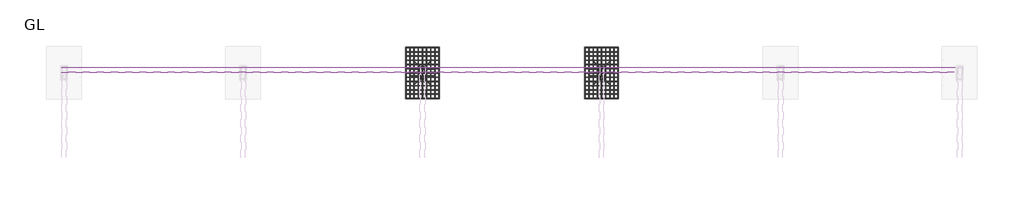
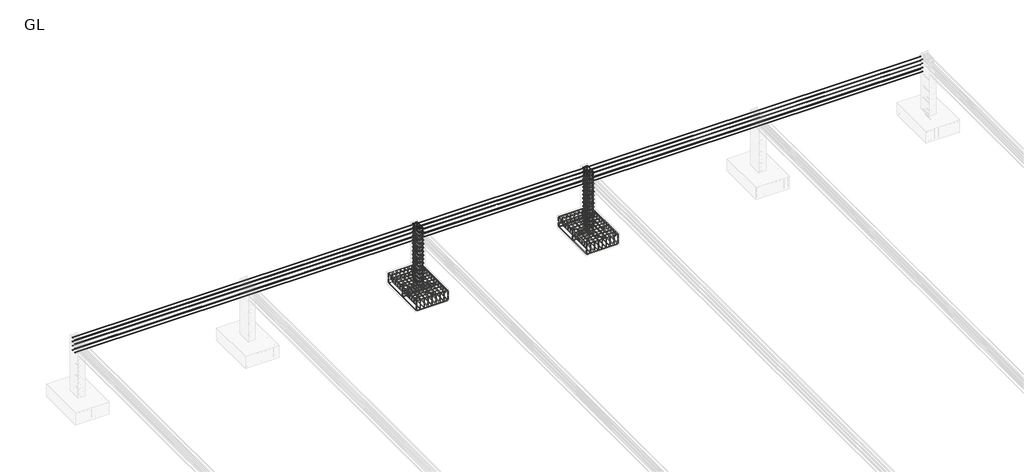
# One storey, part 15 of 16: 23 reinforcing bars.
"""IFC4 building model written with IfcOpenShell, lengths in millimetres."""

from ifc_helpers import new_model, si_unit, point, frame, origin, place, context, project, spatial, polyline, circle_curve, trimmed, segment, composite_curve, source, transform, mapped, element, save
from ifc_brep_helpers import swept_disk

model = new_model("IFC4")

# Units and contexts
model_context = context("Model", 3, world=origin())
ifc_project = project(units=[si_unit("LENGTHUNIT", "METRE", prefix="MILLI")], contexts=[model_context])

# Site, building, storey
site = spatial("IfcSite", under=ifc_project)
building = spatial("IfcBuilding", under=site)
storey = spatial("IfcBuildingStorey", under=building, Name="GL", Elevation=-1829.0)

# Reinforcing bars
placement = place(None, origin())
reinforcing_bar_shape = source(origin(), model_context, "Body", "SolidModel", [
    swept_disk(composite_curve([segment(polyline([(-10050.9544379, 4968.8832479, -2089.0), (-10050.9544379, 4968.8832479, -2213.0)]), True, "CONTINUOUS"), segment(trimmed(circle_curve(frame((-10080.9544379, 4968.8832479, -2213.0), z_axis=(0.0, 1.0, 0.0), x_axis=(30.0, 0.0, 0.0)), 30.0), [point((-10050.9544379, 4968.8832479, -2213.0))], [point((-10080.9544379, 4968.8832479, -2243.0))], True, "CARTESIAN"), True, "CONTINUOUS"), segment(polyline([(-10080.9544379, 4968.8832479, -2243.0), (-11148.9544379, 4968.8832479, -2243.0)]), True, "CONTINUOUS"), segment(trimmed(circle_curve(frame((-11148.9544379, 4968.8832479, -2213.0), z_axis=(0.0, 1.0, 0.0), x_axis=(0.0, 0.0, -30.0)), 30.0), [point((-11148.9544379, 4968.8832479, -2243.0))], [point((-11178.9544379, 4968.8832479, -2213.0))], True, "CARTESIAN"), True, "CONTINUOUS"), segment(polyline([(-11178.9544379, 4968.8832479, -2213.0), (-11178.9544379, 4968.8832479, -2089.0)]), True, "CONTINUOUS")], self_intersect=False), 6.0),
])
element("IfcReinforcingBar", 1, at=placement, inside=storey, context=model_context, shape_type="MappedRepresentation", body=[
    mapped(reinforcing_bar_shape, transform((0.0, 0.0, 0.0), x_axis=(1.0, 0.0, 0.0), y_axis=(0.0, 1.0, 0.0), z_axis=(0.0, 0.0, 1.0))),
    mapped(reinforcing_bar_shape, transform((0.0, -864.0, 0.0), x_axis=(1.0, 0.0, 0.0), y_axis=(0.0, 1.0, 0.0), z_axis=(0.0, 0.0, 1.0))),
    mapped(reinforcing_bar_shape, transform((0.0, -1728.0, 0.0), x_axis=(1.0, 0.0, 0.0), y_axis=(0.0, 1.0, 0.0), z_axis=(0.0, 0.0, 1.0))),
])
reinforcing_bar_2_shape = source(origin(), model_context, "Body", "SolidModel", [
    swept_disk(composite_curve([segment(polyline([(-11178.9544379, 4968.8832479, -2022.436678), (-11178.9544379, 4968.8832479, -1898.436678)]), True, "CONTINUOUS"), segment(trimmed(circle_curve(frame((-11148.9544379, 4968.8832479, -1898.436678), z_axis=(0.0, 1.0, 0.0), x_axis=(-30.0, 0.0, 0.0)), 30.0), [point((-11178.9544379, 4968.8832479, -1898.436678))], [point((-11148.9544379, 4968.8832479, -1868.436678))], True, "CARTESIAN"), True, "CONTINUOUS"), segment(polyline([(-11148.9544379, 4968.8832479, -1868.436678), (-10080.9544379, 4968.8832479, -1868.436678)]), True, "CONTINUOUS"), segment(trimmed(circle_curve(frame((-10080.9544379, 4968.8832479, -1898.436678), z_axis=(0.0, 1.0, 0.0), x_axis=(0.0, 0.0, 30.0)), 30.0), [point((-10080.9544379, 4968.8832479, -1868.436678))], [point((-10050.9544379, 4968.8832479, -1898.436678))], True, "CARTESIAN"), True, "CONTINUOUS"), segment(polyline([(-10050.9544379, 4968.8832479, -1898.436678), (-10050.9544379, 4968.8832479, -2022.436678)]), True, "CONTINUOUS")], self_intersect=False), 6.0),
])
element("IfcReinforcingBar", 2, at=placement, inside=storey, context=model_context, shape_type="MappedRepresentation", body=[
    mapped(reinforcing_bar_2_shape, transform((0.0, 0.0, 0.0), x_axis=(1.0, 0.0, 0.0), y_axis=(0.0, 1.0, 0.0), z_axis=(0.0, 0.0, 1.0))),
    mapped(reinforcing_bar_2_shape, transform((0.0, -144.0, 0.0), x_axis=(1.0, 0.0, 0.0), y_axis=(0.0, 1.0, 0.0), z_axis=(0.0, 0.0, 1.0))),
    mapped(reinforcing_bar_2_shape, transform((0.0, -288.0, 0.0), x_axis=(1.0, 0.0, 0.0), y_axis=(0.0, 1.0, 0.0), z_axis=(0.0, 0.0, 1.0))),
    mapped(reinforcing_bar_2_shape, transform((0.0, -432.0, 0.0), x_axis=(1.0, 0.0, 0.0), y_axis=(0.0, 1.0, 0.0), z_axis=(0.0, 0.0, 1.0))),
    mapped(reinforcing_bar_2_shape, transform((0.0, -576.0, 0.0), x_axis=(1.0, 0.0, 0.0), y_axis=(0.0, 1.0, 0.0), z_axis=(0.0, 0.0, 1.0))),
    mapped(reinforcing_bar_2_shape, transform((0.0, -720.0, 0.0), x_axis=(1.0, 0.0, 0.0), y_axis=(0.0, 1.0, 0.0), z_axis=(0.0, 0.0, 1.0))),
    mapped(reinforcing_bar_2_shape, transform((0.0, -864.0, 0.0), x_axis=(1.0, 0.0, 0.0), y_axis=(0.0, 1.0, 0.0), z_axis=(0.0, 0.0, 1.0))),
    mapped(reinforcing_bar_2_shape, transform((0.0, -1008.0, 0.0), x_axis=(1.0, 0.0, 0.0), y_axis=(0.0, 1.0, 0.0), z_axis=(0.0, 0.0, 1.0))),
    mapped(reinforcing_bar_2_shape, transform((0.0, -1152.0, 0.0), x_axis=(1.0, 0.0, 0.0), y_axis=(0.0, 1.0, 0.0), z_axis=(0.0, 0.0, 1.0))),
    mapped(reinforcing_bar_2_shape, transform((0.0, -1296.0, 0.0), x_axis=(1.0, 0.0, 0.0), y_axis=(0.0, 1.0, 0.0), z_axis=(0.0, 0.0, 1.0))),
    mapped(reinforcing_bar_2_shape, transform((0.0, -1440.0, 0.0), x_axis=(1.0, 0.0, 0.0), y_axis=(0.0, 1.0, 0.0), z_axis=(0.0, 0.0, 1.0))),
    mapped(reinforcing_bar_2_shape, transform((0.0, -1584.0, 0.0), x_axis=(1.0, 0.0, 0.0), y_axis=(0.0, 1.0, 0.0), z_axis=(0.0, 0.0, 1.0))),
    mapped(reinforcing_bar_2_shape, transform((0.0, -1728.0, 0.0), x_axis=(1.0, 0.0, 0.0), y_axis=(0.0, 1.0, 0.0), z_axis=(0.0, 0.0, 1.0))),
])
reinforcing_bar_3_shape = source(origin(), model_context, "Body", "SolidModel", [
    swept_disk(composite_curve([segment(polyline([(-11178.9544379, 3240.8832479, -2027.5081232), (-11178.9544379, 3240.8832479, -1903.5081232)]), True, "CONTINUOUS"), segment(trimmed(circle_curve(frame((-11178.9544379, 3270.8832479, -1903.5081232), z_axis=(-1.0, 0.0, 0.0), x_axis=(0.0, -30.0, 0.0)), 30.0), [point((-11178.9544379, 3240.8832479, -1903.5081232))], [point((-11178.9544379, 3270.8832479, -1873.5081232))], True, "CARTESIAN"), True, "CONTINUOUS"), segment(polyline([(-11178.9544379, 3270.8832479, -1873.5081232), (-11178.9544379, 4938.8832479, -1873.5081232)]), True, "CONTINUOUS"), segment(trimmed(circle_curve(frame((-11178.9544379, 4938.8832479, -1903.5081232), z_axis=(-1.0, 0.0, 0.0), x_axis=(0.0, 0.0, 30.0)), 30.0), [point((-11178.9544379, 4938.8832479, -1873.5081232))], [point((-11178.9544379, 4968.8832479, -1903.5081232))], True, "CARTESIAN"), True, "CONTINUOUS"), segment(polyline([(-11178.9544379, 4968.8832479, -1903.5081232), (-11178.9544379, 4968.8832479, -2027.5081232)]), True, "CONTINUOUS")], self_intersect=False), 6.0),
])
element("IfcReinforcingBar", 3, at=placement, inside=storey, context=model_context, shape_type="MappedRepresentation", body=[
    mapped(reinforcing_bar_3_shape, transform((0.0, 0.0, 0.0), x_axis=(1.0, 0.0, 0.0), y_axis=(0.0, 1.0, 0.0), z_axis=(0.0, 0.0, 1.0))),
    mapped(reinforcing_bar_3_shape, transform((141.0, 0.0, 0.0), x_axis=(1.0, 0.0, 0.0), y_axis=(0.0, 1.0, 0.0), z_axis=(0.0, 0.0, 1.0))),
    mapped(reinforcing_bar_3_shape, transform((282.0, 0.0, 0.0), x_axis=(1.0, 0.0, 0.0), y_axis=(0.0, 1.0, 0.0), z_axis=(0.0, 0.0, 1.0))),
    mapped(reinforcing_bar_3_shape, transform((423.0, 0.0, 0.0), x_axis=(1.0, 0.0, 0.0), y_axis=(0.0, 1.0, 0.0), z_axis=(0.0, 0.0, 1.0))),
    mapped(reinforcing_bar_3_shape, transform((564.0, 0.0, 0.0), x_axis=(1.0, 0.0, 0.0), y_axis=(0.0, 1.0, 0.0), z_axis=(0.0, 0.0, 1.0))),
    mapped(reinforcing_bar_3_shape, transform((705.0, 0.0, 0.0), x_axis=(1.0, 0.0, 0.0), y_axis=(0.0, 1.0, 0.0), z_axis=(0.0, 0.0, 1.0))),
    mapped(reinforcing_bar_3_shape, transform((846.0, 0.0, 0.0), x_axis=(1.0, 0.0, 0.0), y_axis=(0.0, 1.0, 0.0), z_axis=(0.0, 0.0, 1.0))),
    mapped(reinforcing_bar_3_shape, transform((987.0, 0.0, 0.0), x_axis=(1.0, 0.0, 0.0), y_axis=(0.0, 1.0, 0.0), z_axis=(0.0, 0.0, 1.0))),
    mapped(reinforcing_bar_3_shape, transform((1128.0, 0.0, 0.0), x_axis=(1.0, 0.0, 0.0), y_axis=(0.0, 1.0, 0.0), z_axis=(0.0, 0.0, 1.0))),
])
reinforcing_bar_4_shape = source(origin(), model_context, "Body", "SolidModel", [
    swept_disk(composite_curve([segment(polyline([(-10050.9544379, 3240.8832479, -2080.6239909), (-10050.9544379, 3240.8832479, -2204.6239909)]), True, "CONTINUOUS"), segment(trimmed(circle_curve(frame((-10050.9544379, 3270.8832479, -2204.6239909), z_axis=(1.0, 0.0, 0.0), x_axis=(0.0, -30.0, 0.0)), 30.0), [point((-10050.9544379, 3240.8832479, -2204.6239909))], [point((-10050.9544379, 3270.8832479, -2234.6239909))], True, "CARTESIAN"), True, "CONTINUOUS"), segment(polyline([(-10050.9544379, 3270.8832479, -2234.6239909), (-10050.9544379, 4925.8578108, -2234.6239909)]), True, "CONTINUOUS"), segment(trimmed(circle_curve(frame((-10050.9544379, 4925.8578108, -2204.6239909), z_axis=(1.0, 0.0, 0.0), x_axis=(0.0, 0.0, -30.0)), 30.0), [point((-10050.9544379, 4925.8578108, -2234.6239909))], [point((-10050.9544379, 4955.8578108, -2204.6239909))], True, "CARTESIAN"), True, "CONTINUOUS"), segment(polyline([(-10050.9544379, 4955.8578108, -2204.6239909), (-10050.9544379, 4955.8578108, -2080.6239909)]), True, "CONTINUOUS")], self_intersect=False), 6.0),
])
element("IfcReinforcingBar", 4, at=placement, inside=storey, context=model_context, shape_type="MappedRepresentation", body=[
    mapped(reinforcing_bar_4_shape, transform((0.0, 0.0, 0.0), x_axis=(1.0, 0.0, 0.0), y_axis=(0.0, 1.0, 0.0), z_axis=(0.0, 0.0, 1.0))),
    mapped(reinforcing_bar_4_shape, transform((-141.0, 0.0, 0.0), x_axis=(1.0, 0.0, 0.0), y_axis=(0.0, 1.0, 0.0), z_axis=(0.0, 0.0, 1.0))),
    mapped(reinforcing_bar_4_shape, transform((-282.0, 0.0, 0.0), x_axis=(1.0, 0.0, 0.0), y_axis=(0.0, 1.0, 0.0), z_axis=(0.0, 0.0, 1.0))),
    mapped(reinforcing_bar_4_shape, transform((-423.0, 0.0, 0.0), x_axis=(1.0, 0.0, 0.0), y_axis=(0.0, 1.0, 0.0), z_axis=(0.0, 0.0, 1.0))),
    mapped(reinforcing_bar_4_shape, transform((-564.0, 0.0, 0.0), x_axis=(1.0, 0.0, 0.0), y_axis=(0.0, 1.0, 0.0), z_axis=(0.0, 0.0, 1.0))),
    mapped(reinforcing_bar_4_shape, transform((-705.0, 0.0, 0.0), x_axis=(1.0, 0.0, 0.0), y_axis=(0.0, 1.0, 0.0), z_axis=(0.0, 0.0, 1.0))),
    mapped(reinforcing_bar_4_shape, transform((-846.0, 0.0, 0.0), x_axis=(1.0, 0.0, 0.0), y_axis=(0.0, 1.0, 0.0), z_axis=(0.0, 0.0, 1.0))),
    mapped(reinforcing_bar_4_shape, transform((-987.0, 0.0, 0.0), x_axis=(1.0, 0.0, 0.0), y_axis=(0.0, 1.0, 0.0), z_axis=(0.0, 0.0, 1.0))),
    mapped(reinforcing_bar_4_shape, transform((-1128.0, 0.0, 0.0), x_axis=(1.0, 0.0, 0.0), y_axis=(0.0, 1.0, 0.0), z_axis=(0.0, 0.0, 1.0))),
])
reinforcing_bar_5_shape = source(origin(), model_context, "Body", "SolidModel", [
    swept_disk(composite_curve([segment(polyline([(-3954.9544379, 4968.8832479, -2089.0), (-3954.9544379, 4968.8832479, -2213.0)]), True, "CONTINUOUS"), segment(trimmed(circle_curve(frame((-3984.9544379, 4968.8832479, -2213.0), z_axis=(0.0, 1.0, 0.0), x_axis=(30.0, 0.0, 0.0)), 30.0), [point((-3954.9544379, 4968.8832479, -2213.0))], [point((-3984.9544379, 4968.8832479, -2243.0))], True, "CARTESIAN"), True, "CONTINUOUS"), segment(polyline([(-3984.9544379, 4968.8832479, -2243.0), (-5052.9544379, 4968.8832479, -2243.0)]), True, "CONTINUOUS"), segment(trimmed(circle_curve(frame((-5052.9544379, 4968.8832479, -2213.0), z_axis=(0.0, 1.0, 0.0), x_axis=(0.0, 0.0, -30.0)), 30.0), [point((-5052.9544379, 4968.8832479, -2243.0))], [point((-5082.9544379, 4968.8832479, -2213.0))], True, "CARTESIAN"), True, "CONTINUOUS"), segment(polyline([(-5082.9544379, 4968.8832479, -2213.0), (-5082.9544379, 4968.8832479, -2089.0)]), True, "CONTINUOUS")], self_intersect=False), 6.0),
])
element("IfcReinforcingBar", 5, at=placement, inside=storey, context=model_context, shape_type="MappedRepresentation", body=[
    mapped(reinforcing_bar_5_shape, transform((0.0, 0.0, 0.0), x_axis=(1.0, 0.0, 0.0), y_axis=(0.0, 1.0, 0.0), z_axis=(0.0, 0.0, 1.0))),
    mapped(reinforcing_bar_5_shape, transform((0.0, -864.0, 0.0), x_axis=(1.0, 0.0, 0.0), y_axis=(0.0, 1.0, 0.0), z_axis=(0.0, 0.0, 1.0))),
    mapped(reinforcing_bar_5_shape, transform((0.0, -1728.0, 0.0), x_axis=(1.0, 0.0, 0.0), y_axis=(0.0, 1.0, 0.0), z_axis=(0.0, 0.0, 1.0))),
])
reinforcing_bar_6_shape = source(origin(), model_context, "Body", "SolidModel", [
    swept_disk(composite_curve([segment(polyline([(-5082.9544379, 4968.8832479, -2022.436678), (-5082.9544379, 4968.8832479, -1898.436678)]), True, "CONTINUOUS"), segment(trimmed(circle_curve(frame((-5052.9544379, 4968.8832479, -1898.436678), z_axis=(0.0, 1.0, 0.0), x_axis=(-30.0, 0.0, 0.0)), 30.0), [point((-5082.9544379, 4968.8832479, -1898.436678))], [point((-5052.9544379, 4968.8832479, -1868.436678))], True, "CARTESIAN"), True, "CONTINUOUS"), segment(polyline([(-5052.9544379, 4968.8832479, -1868.436678), (-3984.9544379, 4968.8832479, -1868.436678)]), True, "CONTINUOUS"), segment(trimmed(circle_curve(frame((-3984.9544379, 4968.8832479, -1898.436678), z_axis=(0.0, 1.0, 0.0), x_axis=(0.0, 0.0, 30.0)), 30.0), [point((-3984.9544379, 4968.8832479, -1868.436678))], [point((-3954.9544379, 4968.8832479, -1898.436678))], True, "CARTESIAN"), True, "CONTINUOUS"), segment(polyline([(-3954.9544379, 4968.8832479, -1898.436678), (-3954.9544379, 4968.8832479, -2022.436678)]), True, "CONTINUOUS")], self_intersect=False), 6.0),
])
element("IfcReinforcingBar", 6, at=placement, inside=storey, context=model_context, shape_type="MappedRepresentation", body=[
    mapped(reinforcing_bar_6_shape, transform((0.0, 0.0, 0.0), x_axis=(1.0, 0.0, 0.0), y_axis=(0.0, 1.0, 0.0), z_axis=(0.0, 0.0, 1.0))),
    mapped(reinforcing_bar_6_shape, transform((0.0, -144.0, 0.0), x_axis=(1.0, 0.0, 0.0), y_axis=(0.0, 1.0, 0.0), z_axis=(0.0, 0.0, 1.0))),
    mapped(reinforcing_bar_6_shape, transform((0.0, -288.0, 0.0), x_axis=(1.0, 0.0, 0.0), y_axis=(0.0, 1.0, 0.0), z_axis=(0.0, 0.0, 1.0))),
    mapped(reinforcing_bar_6_shape, transform((0.0, -432.0, 0.0), x_axis=(1.0, 0.0, 0.0), y_axis=(0.0, 1.0, 0.0), z_axis=(0.0, 0.0, 1.0))),
    mapped(reinforcing_bar_6_shape, transform((0.0, -576.0, 0.0), x_axis=(1.0, 0.0, 0.0), y_axis=(0.0, 1.0, 0.0), z_axis=(0.0, 0.0, 1.0))),
    mapped(reinforcing_bar_6_shape, transform((0.0, -720.0, 0.0), x_axis=(1.0, 0.0, 0.0), y_axis=(0.0, 1.0, 0.0), z_axis=(0.0, 0.0, 1.0))),
    mapped(reinforcing_bar_6_shape, transform((0.0, -864.0, 0.0), x_axis=(1.0, 0.0, 0.0), y_axis=(0.0, 1.0, 0.0), z_axis=(0.0, 0.0, 1.0))),
    mapped(reinforcing_bar_6_shape, transform((0.0, -1008.0, 0.0), x_axis=(1.0, 0.0, 0.0), y_axis=(0.0, 1.0, 0.0), z_axis=(0.0, 0.0, 1.0))),
    mapped(reinforcing_bar_6_shape, transform((0.0, -1152.0, 0.0), x_axis=(1.0, 0.0, 0.0), y_axis=(0.0, 1.0, 0.0), z_axis=(0.0, 0.0, 1.0))),
    mapped(reinforcing_bar_6_shape, transform((0.0, -1296.0, 0.0), x_axis=(1.0, 0.0, 0.0), y_axis=(0.0, 1.0, 0.0), z_axis=(0.0, 0.0, 1.0))),
    mapped(reinforcing_bar_6_shape, transform((0.0, -1440.0, 0.0), x_axis=(1.0, 0.0, 0.0), y_axis=(0.0, 1.0, 0.0), z_axis=(0.0, 0.0, 1.0))),
    mapped(reinforcing_bar_6_shape, transform((0.0, -1584.0, 0.0), x_axis=(1.0, 0.0, 0.0), y_axis=(0.0, 1.0, 0.0), z_axis=(0.0, 0.0, 1.0))),
    mapped(reinforcing_bar_6_shape, transform((0.0, -1728.0, 0.0), x_axis=(1.0, 0.0, 0.0), y_axis=(0.0, 1.0, 0.0), z_axis=(0.0, 0.0, 1.0))),
])
reinforcing_bar_7_shape = source(origin(), model_context, "Body", "SolidModel", [
    swept_disk(composite_curve([segment(polyline([(-5082.9544379, 3240.8832479, -2027.5081232), (-5082.9544379, 3240.8832479, -1903.5081232)]), True, "CONTINUOUS"), segment(trimmed(circle_curve(frame((-5082.9544379, 3270.8832479, -1903.5081232), z_axis=(-1.0, 0.0, 0.0), x_axis=(0.0, -30.0, 0.0)), 30.0), [point((-5082.9544379, 3240.8832479, -1903.5081232))], [point((-5082.9544379, 3270.8832479, -1873.5081232))], True, "CARTESIAN"), True, "CONTINUOUS"), segment(polyline([(-5082.9544379, 3270.8832479, -1873.5081232), (-5082.9544379, 4938.8832479, -1873.5081232)]), True, "CONTINUOUS"), segment(trimmed(circle_curve(frame((-5082.9544379, 4938.8832479, -1903.5081232), z_axis=(-1.0, 0.0, 0.0), x_axis=(0.0, 0.0, 30.0)), 30.0), [point((-5082.9544379, 4938.8832479, -1873.5081232))], [point((-5082.9544379, 4968.8832479, -1903.5081232))], True, "CARTESIAN"), True, "CONTINUOUS"), segment(polyline([(-5082.9544379, 4968.8832479, -1903.5081232), (-5082.9544379, 4968.8832479, -2027.5081232)]), True, "CONTINUOUS")], self_intersect=False), 6.0),
])
element("IfcReinforcingBar", 7, at=placement, inside=storey, context=model_context, shape_type="MappedRepresentation", body=[
    mapped(reinforcing_bar_7_shape, transform((0.0, 0.0, 0.0), x_axis=(1.0, 0.0, 0.0), y_axis=(0.0, 1.0, 0.0), z_axis=(0.0, 0.0, 1.0))),
    mapped(reinforcing_bar_7_shape, transform((141.0, 0.0, 0.0), x_axis=(1.0, 0.0, 0.0), y_axis=(0.0, 1.0, 0.0), z_axis=(0.0, 0.0, 1.0))),
    mapped(reinforcing_bar_7_shape, transform((282.0, 0.0, 0.0), x_axis=(1.0, 0.0, 0.0), y_axis=(0.0, 1.0, 0.0), z_axis=(0.0, 0.0, 1.0))),
    mapped(reinforcing_bar_7_shape, transform((423.0, 0.0, 0.0), x_axis=(1.0, 0.0, 0.0), y_axis=(0.0, 1.0, 0.0), z_axis=(0.0, 0.0, 1.0))),
    mapped(reinforcing_bar_7_shape, transform((564.0, 0.0, 0.0), x_axis=(1.0, 0.0, 0.0), y_axis=(0.0, 1.0, 0.0), z_axis=(0.0, 0.0, 1.0))),
    mapped(reinforcing_bar_7_shape, transform((705.0, 0.0, 0.0), x_axis=(1.0, 0.0, 0.0), y_axis=(0.0, 1.0, 0.0), z_axis=(0.0, 0.0, 1.0))),
    mapped(reinforcing_bar_7_shape, transform((846.0, 0.0, 0.0), x_axis=(1.0, 0.0, 0.0), y_axis=(0.0, 1.0, 0.0), z_axis=(0.0, 0.0, 1.0))),
    mapped(reinforcing_bar_7_shape, transform((987.0, 0.0, 0.0), x_axis=(1.0, 0.0, 0.0), y_axis=(0.0, 1.0, 0.0), z_axis=(0.0, 0.0, 1.0))),
    mapped(reinforcing_bar_7_shape, transform((1128.0, 0.0, 0.0), x_axis=(1.0, 0.0, 0.0), y_axis=(0.0, 1.0, 0.0), z_axis=(0.0, 0.0, 1.0))),
])
reinforcing_bar_8_shape = source(origin(), model_context, "Body", "SolidModel", [
    swept_disk(composite_curve([segment(polyline([(-3954.9544379, 3240.8832479, -2080.6239909), (-3954.9544379, 3240.8832479, -2204.6239909)]), True, "CONTINUOUS"), segment(trimmed(circle_curve(frame((-3954.9544379, 3270.8832479, -2204.6239909), z_axis=(1.0, 0.0, 0.0), x_axis=(0.0, -30.0, 0.0)), 30.0), [point((-3954.9544379, 3240.8832479, -2204.6239909))], [point((-3954.9544379, 3270.8832479, -2234.6239909))], True, "CARTESIAN"), True, "CONTINUOUS"), segment(polyline([(-3954.9544379, 3270.8832479, -2234.6239909), (-3954.9544379, 4925.8578108, -2234.6239909)]), True, "CONTINUOUS"), segment(trimmed(circle_curve(frame((-3954.9544379, 4925.8578108, -2204.6239909), z_axis=(1.0, 0.0, 0.0), x_axis=(0.0, 0.0, -30.0)), 30.0), [point((-3954.9544379, 4925.8578108, -2234.6239909))], [point((-3954.9544379, 4955.8578108, -2204.6239909))], True, "CARTESIAN"), True, "CONTINUOUS"), segment(polyline([(-3954.9544379, 4955.8578108, -2204.6239909), (-3954.9544379, 4955.8578108, -2080.6239909)]), True, "CONTINUOUS")], self_intersect=False), 6.0),
])
element("IfcReinforcingBar", 8, at=placement, inside=storey, context=model_context, shape_type="MappedRepresentation", body=[
    mapped(reinforcing_bar_8_shape, transform((0.0, 0.0, 0.0), x_axis=(1.0, 0.0, 0.0), y_axis=(0.0, 1.0, 0.0), z_axis=(0.0, 0.0, 1.0))),
    mapped(reinforcing_bar_8_shape, transform((-141.0, 0.0, 0.0), x_axis=(1.0, 0.0, 0.0), y_axis=(0.0, 1.0, 0.0), z_axis=(0.0, 0.0, 1.0))),
    mapped(reinforcing_bar_8_shape, transform((-282.0, 0.0, 0.0), x_axis=(1.0, 0.0, 0.0), y_axis=(0.0, 1.0, 0.0), z_axis=(0.0, 0.0, 1.0))),
    mapped(reinforcing_bar_8_shape, transform((-423.0, 0.0, 0.0), x_axis=(1.0, 0.0, 0.0), y_axis=(0.0, 1.0, 0.0), z_axis=(0.0, 0.0, 1.0))),
    mapped(reinforcing_bar_8_shape, transform((-564.0, 0.0, 0.0), x_axis=(1.0, 0.0, 0.0), y_axis=(0.0, 1.0, 0.0), z_axis=(0.0, 0.0, 1.0))),
    mapped(reinforcing_bar_8_shape, transform((-705.0, 0.0, 0.0), x_axis=(1.0, 0.0, 0.0), y_axis=(0.0, 1.0, 0.0), z_axis=(0.0, 0.0, 1.0))),
    mapped(reinforcing_bar_8_shape, transform((-846.0, 0.0, 0.0), x_axis=(1.0, 0.0, 0.0), y_axis=(0.0, 1.0, 0.0), z_axis=(0.0, 0.0, 1.0))),
    mapped(reinforcing_bar_8_shape, transform((-987.0, 0.0, 0.0), x_axis=(1.0, 0.0, 0.0), y_axis=(0.0, 1.0, 0.0), z_axis=(0.0, 0.0, 1.0))),
    mapped(reinforcing_bar_8_shape, transform((-1128.0, 0.0, 0.0), x_axis=(1.0, 0.0, 0.0), y_axis=(0.0, 1.0, 0.0), z_axis=(0.0, 0.0, 1.0))),
])
reinforcing_bar_9_shape = source(origin(), model_context, "Body", "SolidModel", [
    swept_disk(composite_curve([segment(polyline([(-10607.4864005, 4029.7776922, -1793.0), (-10695.1676414, 3942.0964514, -1793.0)]), True, "CONTINUOUS"), segment(trimmed(circle_curve(frame((-10673.9544379, 3920.8832479, -1793.0), z_axis=(0.0, 0.0, 1.0), x_axis=(-21.21320349999951, 21.213203500000418, 0.0)), 30.0), [point((-10695.1676414, 3942.0964514, -1793.0))], [point((-10673.9544379, 3890.8832479, -1793.0))], True, "CARTESIAN"), True, "CONTINUOUS"), segment(polyline([(-10673.9544379, 3890.8832479, -1793.0), (-10555.9544379, 3890.8832479, -1793.0)]), True, "CONTINUOUS"), segment(trimmed(circle_curve(frame((-10555.9544379, 3920.8832479, -1793.0), z_axis=(0.0, 0.0, 1.0), x_axis=(0.0, -30.0, 0.0)), 30.0), [point((-10555.9544379, 3890.8832479, -1793.0))], [point((-10525.9544379, 3920.8832479, -1793.0))], True, "CARTESIAN"), True, "CONTINUOUS"), segment(polyline([(-10525.9544379, 3920.8832479, -1793.0), (-10525.9544379, 4288.8832479, -1793.0)]), True, "CONTINUOUS"), segment(trimmed(circle_curve(frame((-10555.8864962, 4288.8832479, -1795.0178916), z_axis=(-0.06726305234213417, 0.0, 0.9977352764083365), x_axis=(29.93205830000079, 0.0, 2.0178915999999845)), 30.0), [point((-10525.9544379, 4288.8832479, -1793.0))], [point((-10555.8864962, 4318.8832479, -1795.0178916))], True, "CARTESIAN"), True, "CONTINUOUS"), segment(polyline([(-10555.8864962, 4318.8832479, -1795.0178916), (-10674.0223796, 4318.8832479, -1802.9821084)]), True, "CONTINUOUS"), segment(trimmed(circle_curve(frame((-10674.0223796, 4288.8832479, -1802.9821084), z_axis=(-0.06726305234213417, 0.0, 0.9977352764083365), x_axis=(0.0, 30.0, 0.0)), 30.0), [point((-10674.0223796, 4318.8832479, -1802.9821084))], [point((-10703.9544379, 4288.8832479, -1805.0))], True, "CARTESIAN"), True, "CONTINUOUS"), segment(polyline([(-10703.9544379, 4288.8832479, -1805.0), (-10703.9544379, 3920.8832479, -1805.0)]), True, "CONTINUOUS"), segment(trimmed(circle_curve(frame((-10673.9544379, 3920.8832479, -1805.0), z_axis=(0.0, 0.0, 1.0), x_axis=(-30.0, 0.0, 0.0)), 30.0), [point((-10703.9544379, 3920.8832479, -1805.0))], [point((-10652.7412345, 3899.6700445, -1805.0))], True, "CARTESIAN"), True, "CONTINUOUS"), segment(polyline([(-10652.7412345, 3899.6700445, -1805.0), (-10565.0599936, 3987.3512854, -1805.0)]), True, "CONTINUOUS")], self_intersect=False), 6.0),
])
element("IfcReinforcingBar", 9, at=placement, inside=storey, context=model_context, shape_type="MappedRepresentation", body=[
    mapped(reinforcing_bar_9_shape, transform((0.0, 0.0, 0.0), x_axis=(1.0, 0.0, 0.0), y_axis=(0.0, 1.0, 0.0), z_axis=(0.0, 0.0, 1.0))),
    mapped(reinforcing_bar_9_shape, transform((0.0, 0.0, 144.8571429), x_axis=(1.0, 0.0, 0.0), y_axis=(0.0, 1.0, 0.0), z_axis=(0.0, 0.0, 1.0))),
    mapped(reinforcing_bar_9_shape, transform((0.0, 0.0, 289.7142857), x_axis=(1.0, 0.0, 0.0), y_axis=(0.0, 1.0, 0.0), z_axis=(0.0, 0.0, 1.0))),
    mapped(reinforcing_bar_9_shape, transform((0.0, 0.0, 434.5714286), x_axis=(1.0, 0.0, 0.0), y_axis=(0.0, 1.0, 0.0), z_axis=(0.0, 0.0, 1.0))),
    mapped(reinforcing_bar_9_shape, transform((0.0, 0.0, 579.4285714), x_axis=(1.0, 0.0, 0.0), y_axis=(0.0, 1.0, 0.0), z_axis=(0.0, 0.0, 1.0))),
    mapped(reinforcing_bar_9_shape, transform((0.0, 0.0, 724.2857143), x_axis=(1.0, 0.0, 0.0), y_axis=(0.0, 1.0, 0.0), z_axis=(0.0, 0.0, 1.0))),
    mapped(reinforcing_bar_9_shape, transform((0.0, 0.0, 869.1428571), x_axis=(1.0, 0.0, 0.0), y_axis=(0.0, 1.0, 0.0), z_axis=(0.0, 0.0, 1.0))),
    mapped(reinforcing_bar_9_shape, transform((0.0, 0.0, 1014.0), x_axis=(1.0, 0.0, 0.0), y_axis=(0.0, 1.0, 0.0), z_axis=(0.0, 0.0, 1.0))),
    mapped(reinforcing_bar_9_shape, transform((0.0, 0.0, 1158.8571429), x_axis=(1.0, 0.0, 0.0), y_axis=(0.0, 1.0, 0.0), z_axis=(0.0, 0.0, 1.0))),
    mapped(reinforcing_bar_9_shape, transform((0.0, 0.0, 1303.7142857), x_axis=(1.0, 0.0, 0.0), y_axis=(0.0, 1.0, 0.0), z_axis=(0.0, 0.0, 1.0))),
    mapped(reinforcing_bar_9_shape, transform((0.0, 0.0, 1448.5714286), x_axis=(1.0, 0.0, 0.0), y_axis=(0.0, 1.0, 0.0), z_axis=(0.0, 0.0, 1.0))),
    mapped(reinforcing_bar_9_shape, transform((0.0, 0.0, 1593.4285714), x_axis=(1.0, 0.0, 0.0), y_axis=(0.0, 1.0, 0.0), z_axis=(0.0, 0.0, 1.0))),
    mapped(reinforcing_bar_9_shape, transform((0.0, 0.0, 1738.2857143), x_axis=(1.0, 0.0, 0.0), y_axis=(0.0, 1.0, 0.0), z_axis=(0.0, 0.0, 1.0))),
    mapped(reinforcing_bar_9_shape, transform((0.0, 0.0, 1883.1428571), x_axis=(1.0, 0.0, 0.0), y_axis=(0.0, 1.0, 0.0), z_axis=(0.0, 0.0, 1.0))),
    mapped(reinforcing_bar_9_shape, transform((0.0, 0.0, 2028.0), x_axis=(1.0, 0.0, 0.0), y_axis=(0.0, 1.0, 0.0), z_axis=(0.0, 0.0, 1.0))),
])
element("IfcReinforcingBar", 10, at=placement, inside=storey, context=model_context, shape_type="SolidModel", body=[
    swept_disk(composite_curve([segment(polyline([(-10672.0642232, 3919.9357561, 241.0), (-10672.0642232, 3919.9357561, -2129.0)]), True, "CONTINUOUS"), segment(trimmed(circle_curve(frame((-10693.2774266, 3898.7225527, -2129.0), z_axis=(-0.7071067811865187, 0.7071067811865764, 0.0), x_axis=(21.213203400000566, 21.21320340000011, 0.0)), 30.0), [point((-10672.0642232, 3919.9357561, -2129.0))], [point((-10693.2774266, 3898.7225527, -2159.0))], True, "CARTESIAN"), True, "CONTINUOUS"), segment(polyline([(-10693.2774266, 3898.7225527, -2159.0), (-10940.7648, 3651.2351793, -2159.0)]), True, "CONTINUOUS")], self_intersect=False), 6.0),
])
element("IfcReinforcingBar", 11, at=placement, inside=storey, context=model_context, shape_type="SolidModel", body=[
    swept_disk(composite_curve([segment(polyline([(-10672.0642232, 4289.8307397, 241.0), (-10672.0642232, 4289.8307397, -2129.0)]), True, "CONTINUOUS"), segment(trimmed(circle_curve(frame((-10693.2774266, 4311.0439432, -2129.0), z_axis=(0.7071067811865218, 0.7071067811865733, 0.0), x_axis=(21.213203400000566, -21.213203500000418, 0.0)), 30.0), [point((-10672.0642232, 4289.8307397, -2129.0))], [point((-10693.2774266, 4311.0439432, -2159.0))], True, "CARTESIAN"), True, "CONTINUOUS"), segment(polyline([(-10693.2774266, 4311.0439432, -2159.0), (-10940.7648, 4558.5313166, -2159.0)]), True, "CONTINUOUS")], self_intersect=False), 6.0),
])
element("IfcReinforcingBar", 12, at=placement, inside=storey, context=model_context, shape_type="SolidModel", body=[
    swept_disk(composite_curve([segment(polyline([(-10557.8446527, 3919.9357561, 241.0), (-10557.8446527, 3919.9357561, -2129.0)]), True, "CONTINUOUS"), segment(trimmed(circle_curve(frame((-10536.6314492, 3898.7225527, -2129.0), z_axis=(-0.7071067811865248, -0.7071067811865703, 0.0), x_axis=(-21.21320349999951, 21.21320340000011, 0.0)), 30.0), [point((-10557.8446527, 3919.9357561, -2129.0))], [point((-10536.6314492, 3898.7225527, -2159.0))], True, "CARTESIAN"), True, "CONTINUOUS"), segment(polyline([(-10536.6314492, 3898.7225527, -2159.0), (-10289.1440758, 3651.2351793, -2159.0)]), True, "CONTINUOUS")], self_intersect=False), 6.0),
])
element("IfcReinforcingBar", 13, at=placement, inside=storey, context=model_context, shape_type="SolidModel", body=[
    swept_disk(composite_curve([segment(polyline([(-10557.8446527, 4289.8307397, 241.0), (-10557.8446527, 4289.8307397, -2129.0)]), True, "CONTINUOUS"), segment(trimmed(circle_curve(frame((-10536.6314492, 4311.0439432, -2129.0), z_axis=(0.7071067811865157, -0.7071067811865794, 0.0), x_axis=(-21.21320349999951, -21.213203500000418, 0.0)), 30.0), [point((-10557.8446527, 4289.8307397, -2129.0))], [point((-10536.6314492, 4311.0439432, -2159.0))], True, "CARTESIAN"), True, "CONTINUOUS"), segment(polyline([(-10536.6314492, 4311.0439432, -2159.0), (-10289.1440758, 4558.5313166, -2159.0)]), True, "CONTINUOUS")], self_intersect=False), 6.0),
])
reinforcing_bar_10_shape = source(origin(), model_context, "Body", "SolidModel", [
    swept_disk(composite_curve([segment(polyline([(-10672.0642232, 3997.0882595, 241.0), (-10672.0642232, 3997.0882595, -2129.0)]), True, "CONTINUOUS"), segment(trimmed(circle_curve(frame((-10702.0642232, 3997.0882595, -2129.0), z_axis=(0.0, 1.0, 0.0), x_axis=(30.0, 0.0, 0.0)), 30.0), [point((-10672.0642232, 3997.0882595, -2129.0))], [point((-10702.0642232, 3997.0882595, -2159.0))], True, "CARTESIAN"), True, "CONTINUOUS"), segment(polyline([(-10702.0642232, 3997.0882595, -2159.0), (-11052.0642232, 3997.0882595, -2159.0)]), True, "CONTINUOUS")], self_intersect=False), 6.0),
])
element("IfcReinforcingBar", 14, at=placement, inside=storey, context=model_context, shape_type="MappedRepresentation", body=[
    mapped(reinforcing_bar_10_shape, transform((0.0, 0.0, 0.0), x_axis=(1.0, 0.0, 0.0), y_axis=(0.0, 1.0, 0.0), z_axis=(0.0, 0.0, 1.0))),
    mapped(reinforcing_bar_10_shape, transform((0.0, 123.5823926, 0.0), x_axis=(1.0, 0.0, 0.0), y_axis=(0.0, 1.0, 0.0), z_axis=(0.0, 0.0, 1.0))),
    mapped(reinforcing_bar_10_shape, transform((0.0, 247.1647853, 0.0), x_axis=(1.0, 0.0, 0.0), y_axis=(0.0, 1.0, 0.0), z_axis=(0.0, 0.0, 1.0))),
])
reinforcing_bar_11_shape = source(origin(), model_context, "Body", "SolidModel", [
    swept_disk(composite_curve([segment(polyline([(-10557.8446527, 3997.0882595, 241.0), (-10557.8446527, 3997.0882595, -2129.0)]), True, "CONTINUOUS"), segment(trimmed(circle_curve(frame((-10527.8446527, 3997.0882595, -2129.0), z_axis=(0.0, -1.0, 0.0), x_axis=(-30.0, 0.0, 0.0)), 30.0), [point((-10557.8446527, 3997.0882595, -2129.0))], [point((-10527.8446527, 3997.0882595, -2159.0))], True, "CARTESIAN"), True, "CONTINUOUS"), segment(polyline([(-10527.8446527, 3997.0882595, -2159.0), (-10177.8446527, 3997.0882595, -2159.0)]), True, "CONTINUOUS")], self_intersect=False), 6.0),
])
element("IfcReinforcingBar", 15, at=placement, inside=storey, context=model_context, shape_type="MappedRepresentation", body=[
    mapped(reinforcing_bar_11_shape, transform((0.0, 0.0, 0.0), x_axis=(1.0, 0.0, 0.0), y_axis=(0.0, 1.0, 0.0), z_axis=(0.0, 0.0, 1.0))),
    mapped(reinforcing_bar_11_shape, transform((0.0, 123.5823926, 0.0), x_axis=(1.0, 0.0, 0.0), y_axis=(0.0, 1.0, 0.0), z_axis=(0.0, 0.0, 1.0))),
    mapped(reinforcing_bar_11_shape, transform((0.0, 247.1647853, 0.0), x_axis=(1.0, 0.0, 0.0), y_axis=(0.0, 1.0, 0.0), z_axis=(0.0, 0.0, 1.0))),
])
reinforcing_bar_12_shape = source(origin(), model_context, "Body", "SolidModel", [
    swept_disk(composite_curve([segment(polyline([(-4511.4864005, 4029.7776922, -1793.0), (-4599.1676414, 3942.0964514, -1793.0)]), True, "CONTINUOUS"), segment(trimmed(circle_curve(frame((-4577.9544379, 3920.8832479, -1793.0), z_axis=(0.0, 0.0, 1.0), x_axis=(-21.213203500000418, 21.213203500000418, 0.0)), 30.0), [point((-4599.1676414, 3942.0964514, -1793.0))], [point((-4577.9544379, 3890.8832479, -1793.0))], True, "CARTESIAN"), True, "CONTINUOUS"), segment(polyline([(-4577.9544379, 3890.8832479, -1793.0), (-4459.9544379, 3890.8832479, -1793.0)]), True, "CONTINUOUS"), segment(trimmed(circle_curve(frame((-4459.9544379, 3920.8832479, -1793.0), z_axis=(0.0, 0.0, 1.0), x_axis=(0.0, -30.0, 0.0)), 30.0), [point((-4459.9544379, 3890.8832479, -1793.0))], [point((-4429.9544379, 3920.8832479, -1793.0))], True, "CARTESIAN"), True, "CONTINUOUS"), segment(polyline([(-4429.9544379, 3920.8832479, -1793.0), (-4429.9544379, 4288.8832479, -1793.0)]), True, "CONTINUOUS"), segment(trimmed(circle_curve(frame((-4459.8864962, 4288.8832479, -1795.0178916), z_axis=(-0.06726305234213417, 0.0, 0.9977352764083365), x_axis=(29.93205829999988, 0.0, 2.0178915999999845)), 30.0), [point((-4429.9544379, 4288.8832479, -1793.0))], [point((-4459.8864962, 4318.8832479, -1795.0178916))], True, "CARTESIAN"), True, "CONTINUOUS"), segment(polyline([(-4459.8864962, 4318.8832479, -1795.0178916), (-4578.0223796, 4318.8832479, -1802.9821084)]), True, "CONTINUOUS"), segment(trimmed(circle_curve(frame((-4578.0223796, 4288.8832479, -1802.9821084), z_axis=(-0.06726305234213417, 0.0, 0.9977352764083365), x_axis=(0.0, 30.0, 0.0)), 30.0), [point((-4578.0223796, 4318.8832479, -1802.9821084))], [point((-4607.9544379, 4288.8832479, -1805.0))], True, "CARTESIAN"), True, "CONTINUOUS"), segment(polyline([(-4607.9544379, 4288.8832479, -1805.0), (-4607.9544379, 3920.8832479, -1805.0)]), True, "CONTINUOUS"), segment(trimmed(circle_curve(frame((-4577.9544379, 3920.8832479, -1805.0), z_axis=(0.0, 0.0, 1.0), x_axis=(-30.0, 0.0, 0.0)), 30.0), [point((-4607.9544379, 3920.8832479, -1805.0))], [point((-4556.7412345, 3899.6700445, -1805.0))], True, "CARTESIAN"), True, "CONTINUOUS"), segment(polyline([(-4556.7412345, 3899.6700445, -1805.0), (-4469.0599936, 3987.3512854, -1805.0)]), True, "CONTINUOUS")], self_intersect=False), 6.0),
])
element("IfcReinforcingBar", 16, at=placement, inside=storey, context=model_context, shape_type="MappedRepresentation", body=[
    mapped(reinforcing_bar_12_shape, transform((0.0, 0.0, 0.0), x_axis=(1.0, 0.0, 0.0), y_axis=(0.0, 1.0, 0.0), z_axis=(0.0, 0.0, 1.0))),
    mapped(reinforcing_bar_12_shape, transform((0.0, 0.0, 144.8571429), x_axis=(1.0, 0.0, 0.0), y_axis=(0.0, 1.0, 0.0), z_axis=(0.0, 0.0, 1.0))),
    mapped(reinforcing_bar_12_shape, transform((0.0, 0.0, 289.7142857), x_axis=(1.0, 0.0, 0.0), y_axis=(0.0, 1.0, 0.0), z_axis=(0.0, 0.0, 1.0))),
    mapped(reinforcing_bar_12_shape, transform((0.0, 0.0, 434.5714286), x_axis=(1.0, 0.0, 0.0), y_axis=(0.0, 1.0, 0.0), z_axis=(0.0, 0.0, 1.0))),
    mapped(reinforcing_bar_12_shape, transform((0.0, 0.0, 579.4285714), x_axis=(1.0, 0.0, 0.0), y_axis=(0.0, 1.0, 0.0), z_axis=(0.0, 0.0, 1.0))),
    mapped(reinforcing_bar_12_shape, transform((0.0, 0.0, 724.2857143), x_axis=(1.0, 0.0, 0.0), y_axis=(0.0, 1.0, 0.0), z_axis=(0.0, 0.0, 1.0))),
    mapped(reinforcing_bar_12_shape, transform((0.0, 0.0, 869.1428571), x_axis=(1.0, 0.0, 0.0), y_axis=(0.0, 1.0, 0.0), z_axis=(0.0, 0.0, 1.0))),
    mapped(reinforcing_bar_12_shape, transform((0.0, 0.0, 1014.0), x_axis=(1.0, 0.0, 0.0), y_axis=(0.0, 1.0, 0.0), z_axis=(0.0, 0.0, 1.0))),
    mapped(reinforcing_bar_12_shape, transform((0.0, 0.0, 1158.8571429), x_axis=(1.0, 0.0, 0.0), y_axis=(0.0, 1.0, 0.0), z_axis=(0.0, 0.0, 1.0))),
    mapped(reinforcing_bar_12_shape, transform((0.0, 0.0, 1303.7142857), x_axis=(1.0, 0.0, 0.0), y_axis=(0.0, 1.0, 0.0), z_axis=(0.0, 0.0, 1.0))),
    mapped(reinforcing_bar_12_shape, transform((0.0, 0.0, 1448.5714286), x_axis=(1.0, 0.0, 0.0), y_axis=(0.0, 1.0, 0.0), z_axis=(0.0, 0.0, 1.0))),
    mapped(reinforcing_bar_12_shape, transform((0.0, 0.0, 1593.4285714), x_axis=(1.0, 0.0, 0.0), y_axis=(0.0, 1.0, 0.0), z_axis=(0.0, 0.0, 1.0))),
    mapped(reinforcing_bar_12_shape, transform((0.0, 0.0, 1738.2857143), x_axis=(1.0, 0.0, 0.0), y_axis=(0.0, 1.0, 0.0), z_axis=(0.0, 0.0, 1.0))),
    mapped(reinforcing_bar_12_shape, transform((0.0, 0.0, 1883.1428571), x_axis=(1.0, 0.0, 0.0), y_axis=(0.0, 1.0, 0.0), z_axis=(0.0, 0.0, 1.0))),
    mapped(reinforcing_bar_12_shape, transform((0.0, 0.0, 2028.0), x_axis=(1.0, 0.0, 0.0), y_axis=(0.0, 1.0, 0.0), z_axis=(0.0, 0.0, 1.0))),
])
element("IfcReinforcingBar", 17, at=placement, inside=storey, context=model_context, shape_type="SolidModel", body=[
    swept_disk(composite_curve([segment(polyline([(-4576.0642232, 3919.9357561, 241.0), (-4576.0642232, 3919.9357561, -2129.0)]), True, "CONTINUOUS"), segment(trimmed(circle_curve(frame((-4597.2774266, 3898.7225527, -2129.0), z_axis=(-0.7071067811865187, 0.7071067811865764, 0.0), x_axis=(21.213203399999657, 21.21320340000011, 0.0)), 30.0), [point((-4576.0642232, 3919.9357561, -2129.0))], [point((-4597.2774266, 3898.7225527, -2159.0))], True, "CARTESIAN"), True, "CONTINUOUS"), segment(polyline([(-4597.2774266, 3898.7225527, -2159.0), (-4844.7648, 3651.2351793, -2159.0)]), True, "CONTINUOUS")], self_intersect=False), 6.0),
])
element("IfcReinforcingBar", 18, at=placement, inside=storey, context=model_context, shape_type="SolidModel", body=[
    swept_disk(composite_curve([segment(polyline([(-4576.0642232, 4289.8307397, 241.0), (-4576.0642232, 4289.8307397, -2129.0)]), True, "CONTINUOUS"), segment(trimmed(circle_curve(frame((-4597.2774266, 4311.0439432, -2129.0), z_axis=(0.7071067811865218, 0.7071067811865733, 0.0), x_axis=(21.213203399999657, -21.213203500000418, 0.0)), 30.0), [point((-4576.0642232, 4289.8307397, -2129.0))], [point((-4597.2774266, 4311.0439432, -2159.0))], True, "CARTESIAN"), True, "CONTINUOUS"), segment(polyline([(-4597.2774266, 4311.0439432, -2159.0), (-4844.7648, 4558.5313166, -2159.0)]), True, "CONTINUOUS")], self_intersect=False), 6.0),
])
element("IfcReinforcingBar", 19, at=placement, inside=storey, context=model_context, shape_type="SolidModel", body=[
    swept_disk(composite_curve([segment(polyline([(-4461.8446527, 3919.9357561, 241.0), (-4461.8446527, 3919.9357561, -2129.0)]), True, "CONTINUOUS"), segment(trimmed(circle_curve(frame((-4440.6314492, 3898.7225527, -2129.0), z_axis=(-0.7071067811865248, -0.7071067811865703, 0.0), x_axis=(-21.21320349999951, 21.21320340000011, 0.0)), 30.0), [point((-4461.8446527, 3919.9357561, -2129.0))], [point((-4440.6314492, 3898.7225527, -2159.0))], True, "CARTESIAN"), True, "CONTINUOUS"), segment(polyline([(-4440.6314492, 3898.7225527, -2159.0), (-4193.1440758, 3651.2351793, -2159.0)]), True, "CONTINUOUS")], self_intersect=False), 6.0),
])
element("IfcReinforcingBar", 20, at=placement, inside=storey, context=model_context, shape_type="SolidModel", body=[
    swept_disk(composite_curve([segment(polyline([(-4461.8446527, 4289.8307397, 241.0), (-4461.8446527, 4289.8307397, -2129.0)]), True, "CONTINUOUS"), segment(trimmed(circle_curve(frame((-4440.6314492, 4311.0439432, -2129.0), z_axis=(0.7071067811865157, -0.7071067811865794, 0.0), x_axis=(-21.21320349999951, -21.213203500000418, 0.0)), 30.0), [point((-4461.8446527, 4289.8307397, -2129.0))], [point((-4440.6314492, 4311.0439432, -2159.0))], True, "CARTESIAN"), True, "CONTINUOUS"), segment(polyline([(-4440.6314492, 4311.0439432, -2159.0), (-4193.1440758, 4558.5313166, -2159.0)]), True, "CONTINUOUS")], self_intersect=False), 6.0),
])
reinforcing_bar_13_shape = source(origin(), model_context, "Body", "SolidModel", [
    swept_disk(composite_curve([segment(polyline([(-4576.0642232, 3997.0882595, 241.0), (-4576.0642232, 3997.0882595, -2129.0)]), True, "CONTINUOUS"), segment(trimmed(circle_curve(frame((-4606.0642232, 3997.0882595, -2129.0), z_axis=(0.0, 1.0, 0.0), x_axis=(30.0, 0.0, 0.0)), 30.0), [point((-4576.0642232, 3997.0882595, -2129.0))], [point((-4606.0642232, 3997.0882595, -2159.0))], True, "CARTESIAN"), True, "CONTINUOUS"), segment(polyline([(-4606.0642232, 3997.0882595, -2159.0), (-4956.0642232, 3997.0882595, -2159.0)]), True, "CONTINUOUS")], self_intersect=False), 6.0),
])
element("IfcReinforcingBar", 21, at=placement, inside=storey, context=model_context, shape_type="MappedRepresentation", body=[
    mapped(reinforcing_bar_13_shape, transform((0.0, 0.0, 0.0), x_axis=(1.0, 0.0, 0.0), y_axis=(0.0, 1.0, 0.0), z_axis=(0.0, 0.0, 1.0))),
    mapped(reinforcing_bar_13_shape, transform((0.0, 123.5823926, 0.0), x_axis=(1.0, 0.0, 0.0), y_axis=(0.0, 1.0, 0.0), z_axis=(0.0, 0.0, 1.0))),
    mapped(reinforcing_bar_13_shape, transform((0.0, 247.1647853, 0.0), x_axis=(1.0, 0.0, 0.0), y_axis=(0.0, 1.0, 0.0), z_axis=(0.0, 0.0, 1.0))),
])
reinforcing_bar_14_shape = source(origin(), model_context, "Body", "SolidModel", [
    swept_disk(composite_curve([segment(polyline([(7496.2065564, 4288.0653602, 208.2829644), (-22901.9544379, 4288.0653602, 208.2829644)]), True, "CONTINUOUS")], self_intersect=False), 6.0),
])
element("IfcReinforcingBar", 22, at=placement, inside=storey, context=model_context, shape_type="MappedRepresentation", body=[
    mapped(reinforcing_bar_14_shape, transform((0.0, 0.0, 0.0), x_axis=(1.0, 0.0, 0.0), y_axis=(0.0, 1.0, 0.0), z_axis=(0.0, 0.0, 1.0))),
    mapped(reinforcing_bar_14_shape, transform((0.0, 0.0, -155.5868389), x_axis=(1.0, 0.0, 0.0), y_axis=(0.0, 1.0, 0.0), z_axis=(0.0, 0.0, 1.0))),
    mapped(reinforcing_bar_14_shape, transform((0.0, 0.0, -311.1736778), x_axis=(1.0, 0.0, 0.0), y_axis=(0.0, 1.0, 0.0), z_axis=(0.0, 0.0, 1.0))),
    mapped(reinforcing_bar_14_shape, transform((0.0, 0.0, -466.7605167), x_axis=(1.0, 0.0, 0.0), y_axis=(0.0, 1.0, 0.0), z_axis=(0.0, 0.0, 1.0))),
])
reinforcing_bar_15_shape = source(origin(), model_context, "Body", "SolidModel", [
    swept_disk(composite_curve([segment(polyline([(7479.7232994, 4129.4805073, -258.4775522), (-22901.9544379, 4129.4805073, -258.4775522)]), True, "CONTINUOUS")], self_intersect=False), 6.0),
])
element("IfcReinforcingBar", 23, at=placement, inside=storey, context=model_context, shape_type="MappedRepresentation", body=[
    mapped(reinforcing_bar_15_shape, transform((0.0, 0.0, 0.0), x_axis=(1.0, 0.0, 0.0), y_axis=(0.0, 1.0, 0.0), z_axis=(0.0, 0.0, 1.0))),
    mapped(reinforcing_bar_15_shape, transform((0.0, 0.0, 155.5868389), x_axis=(1.0, 0.0, 0.0), y_axis=(0.0, 1.0, 0.0), z_axis=(0.0, 0.0, 1.0))),
    mapped(reinforcing_bar_15_shape, transform((0.0, 0.0, 311.1736778), x_axis=(1.0, 0.0, 0.0), y_axis=(0.0, 1.0, 0.0), z_axis=(0.0, 0.0, 1.0))),
    mapped(reinforcing_bar_15_shape, transform((0.0, 0.0, 466.7605167), x_axis=(1.0, 0.0, 0.0), y_axis=(0.0, 1.0, 0.0), z_axis=(0.0, 0.0, 1.0))),
])

save(model, "model.ifc")

# Revit data of these elements
# Elements 1, 2, 3, 4, 5, 6, 7, 8, 9, 10, 11, 12, 13, 14, 15, 16, 17, 18, 19, 20, 21, 22, 23 (IfcReinforcingBar)
#   Phase Created = New Construction
